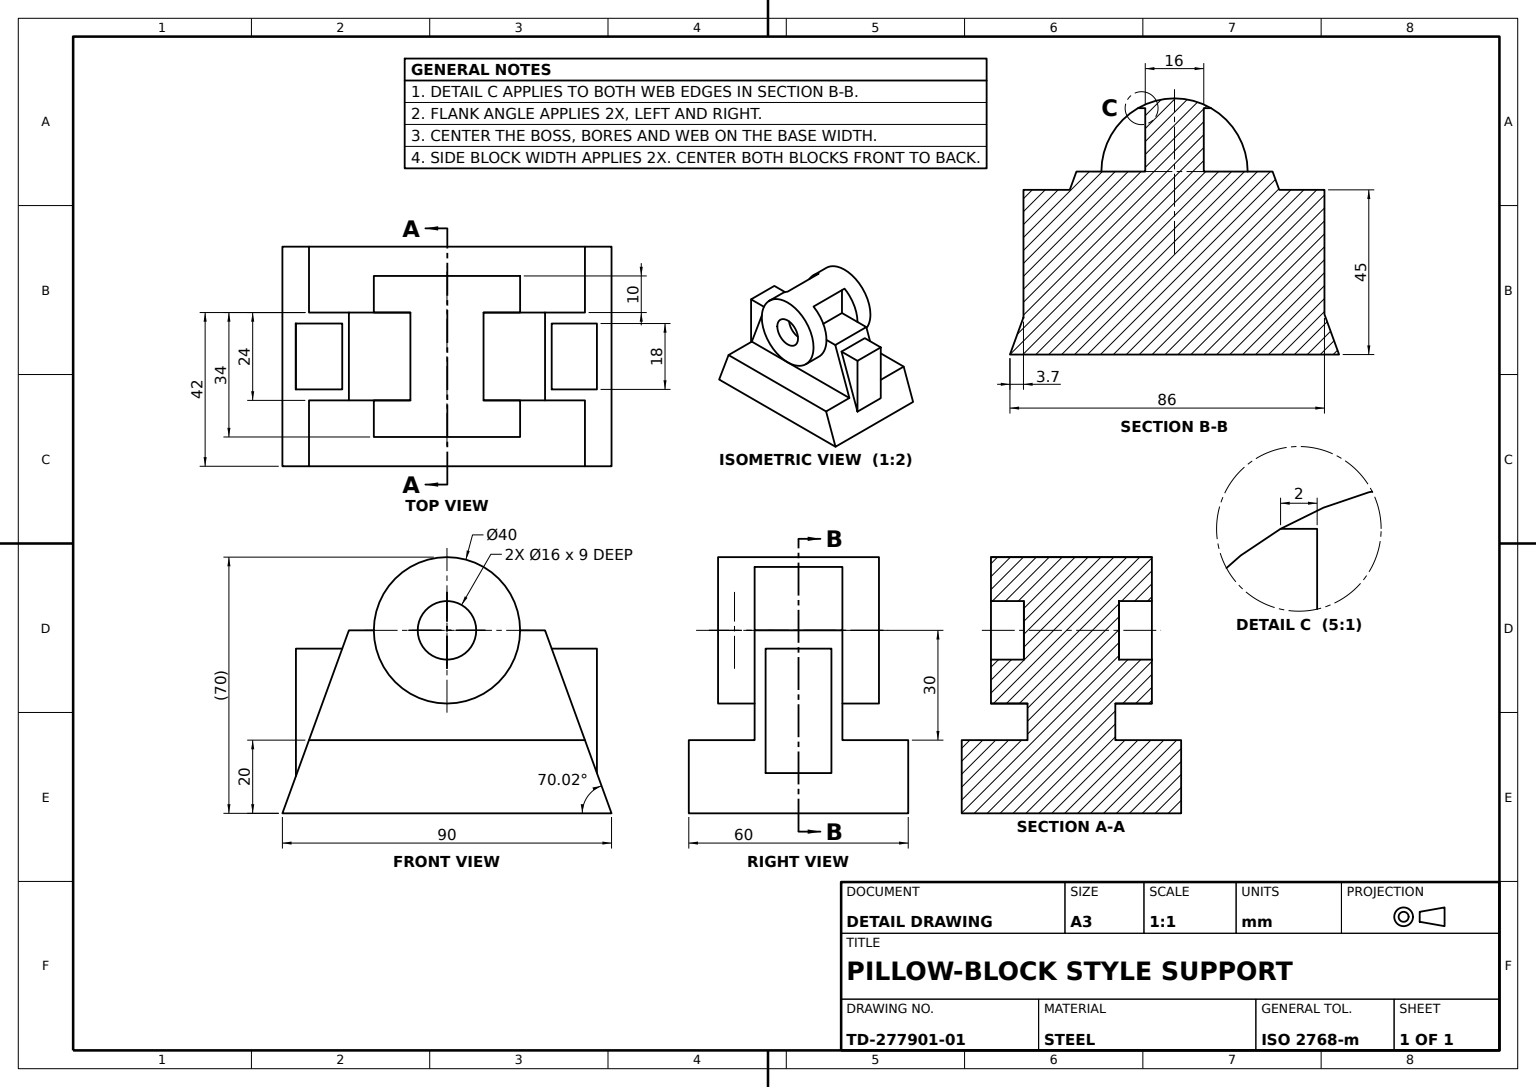
SolidWorks part; units mm, degrees
material "Plain Carbon Steel"
ref_plane "Front Plane" through (0, 0, 0) normal (0, 0, 1) x (1, 0, 0)
ref_plane "Top Plane" through (0, 0, 0) normal (0, 1, 0) x (1, 0, 0)
ref_plane "Right Plane" through (0, 0, 0) normal (1, 0, 0) x (0, 0, -1)
sketch "Base Trapezoid Sketch" plane through (0, 0, 0) normal (0, 0, 1) x (1, 0, 0)
  line L0 (0, 0) -> (90, 0)
  line L1 (90, 0) -> (90, 20)
  line L2 (90, 20) -> (0, 20)
  line L3 (0, 20) -> (0, 0)
  dimension "D1" = 90
  dimension "D2" = 20
extrude "Trapezoid Base" add sketch "Base Trapezoid Sketch" along normal blind 60
sketch "Support Profile Sketch" plane through (0, 0, 60) normal (0, 0, 1) x (1, 0, 0)
  line L0 (45, 20) -> (7.2727, 20)
  line L1 (90, 20) -> (0, 20) construction
  line L2 (45, 55) -> (20, 55)
  line L3 (20, 55) -> (7.2727, 20)
  line L4 (45, 55) -> (70, 55)
  line L5 (70, 55) -> (82.7273, 20)
  line L6 (45, 20) -> (82.7273, 20)
  line L7 (0, 20) -> (0, 0) construction
  line L8 (0, 0) -> (90, 0) construction
  dimension "D1" = 7.2727
  dimension "D2" = 20
  dimension "D3" = 55
extrude "Cylinder Support" add sketch "Support Profile Sketch" against normal blind 42
sketch "Support Notch Sketch" plane through (0, 0, 60) normal (0, 0, 1) x (1, 0, 0)
  line L0 (7.2727, 20) -> (20, 55)
  line L1 (20, 55) -> (70, 55)
  line L2 (70, 55) -> (82.7273, 20)
  line L3 (82.7273, 20) -> (7.2727, 20)
extrude "Support Notch Cut" cut sketch "Support Notch Sketch" against normal blind 18
sketch "Support Relief Sketch" plane through (0, 0, 42) normal (0, 0, 1) x (1, 0, 0)
  line L2 (45, 50) -> (71.8182, 50)
  line L3 (82.7273, 20) -> (70, 55) construction
  line L5 (45, 50) -> (18.1818, 50)
  line L6 (20, 55) -> (7.2727, 20) construction
  line L7 (18.1818, 50) -> (20, 55)
  line L8 (20, 55) -> (70, 55)
  line L9 (70, 55) -> (20, 55) construction
  line L10 (70, 55) -> (71.8182, 50)
  dimension "D1" = 10.9091
extrude "Support Relief Cut" cut sketch "Support Relief Sketch" against normal blind 24
sketch "Through Profile Sketch" plane through (0, 0, 60) normal (0, 0, 1) x (1, 0, 0)
  line L0 (0, 20) -> (7.2727, 20)
  line L1 (0, 20) -> (0, 0) construction
  line L2 (7.2727, 20) -> (0, 0)
  line L3 (90, 20) -> (82.7273, 20)
  line L4 (82.7273, 20) -> (90, 0)
  line L5 (90, 0) -> (90, 20)
  line M1 (90, 20) -> (0, 20)
  line M2 (0, 20) -> (0, 0)
  line M4 (90, 0) -> (90, 20)
extrude "Through Profile Cut" cut sketch "Through Profile Sketch" against normal blind 60 contours L2 M1 M2 | L4 M1 M4
sketch "Cylinder Sketch Ø40" plane through (0, 0, 42) normal (0, 0, 1) x (1, 0, 0)
  line L0 (18.1818, 50) -> (71.8182, 50) construction
  circle A0 centre (45, 50) radius 20
  dimension "D1" = 40
  dimension "D2" = 40
extrude "Cylinder Ø40" add sketch "Cylinder Sketch Ø40" against normal blind 34
sketch "Cylinder Extension Sketch" plane through (0, 0, 42) normal (0, 0, 1) x (1, 0, 0)
  circle A0 centre (45, 50) radius 20
  dimension "D1" = 40
  dimension "D2" = 40
extrude "Cylinder Extension Ø40" add sketch "Cylinder Extension Sketch" along normal blind 10
sketch "Front Bore Sketch Ø16" plane through (0, 0, 52) normal (0, 0, 1) x (1, 0, 0)
  circle A0 centre (45, 50) radius 8
  dimension "D1" = 16
  dimension "D2" = 16
extrude "Front Bore Ø16" cut sketch "Front Bore Sketch Ø16" against normal blind 10
sketch "Rear Bore Sketch" plane through (0, 0, 8) normal (0, 0, -1) x (-1, 0, 0)
  circle A0 centre (-45, 50) radius 8
  dimension "D1" = 16
extrude "Rear Bore" cut sketch "Rear Bore Sketch" against normal blind 10
ref_plane "Side Block Plane" through (0, 0, 0) normal (1, 0, 0) x (0, 0, -1)
sketch "Side Block Sketch" plane through (0, 0, 0) normal (1, 0, 0) x (0, 0, -1)
  line L2 (-30, 45) -> (-39, 45)
  line L3 (-39, 45) -> (-39, 10)
  line L4 (-39, 10) -> (-21, 10)
  line L5 (-21, 10) -> (-21, 45)
  line L6 (-21, 45) -> (-30, 45)
  dimension "D1" = 18
  dimension "D2" = 35
  dimension "D3" = 30
  dimension "D4" = 10
extrude "Side Blocks" add sketch "Side Block Sketch" along normal blind 86
sketch "Block Trim Sketch" plane through (0, 0, 0) normal (-1, 0, 0) x (0, 0, 1)
  line L0 (21, 45) -> (39, 45)
  line L1 (39, 45) -> (39, 10)
  line L2 (39, 10) -> (21, 10)
  line L3 (21, 10) -> (21, 45)
extrude "Block Trim Cut" cut sketch "Block Trim Sketch" against normal blind 3.7
ref_plane "Plane2" through (0, 50, 0) normal (0, 1, 0) x (1, 0, 0)
ref_plane "4" through (0, 70, 0) normal (0, 1, 0) x (1, 0, 0)
ref_plane "Plane4" through (0, 65, 0) normal (0, 1, 0) x (1, 0, 0)
ref_plane "Plane5" through (0, 50, 0) normal (0, 1, 0) x (1, 0, 0)
ref_plane "Slot A Plane" through (65, 0, 0) normal (1, 0, 0) x (0, 0, -1)
sketch "Slot A Sketch" plane through (65, 0, 0) normal (1, 0, 0) x (0, 0, -1)
  line L2 (-8, 70) -> (-52, 70) construction
  line L3 (-42, 70) -> (-18, 70)
  line L4 (-18, 70) -> (-18, 50)
  line L5 (-18, 50) -> (-42, 50)
  line L6 (-42, 70) -> (-42, 50)
extrude "Slot A Cut" cut sketch "Slot A Sketch" against normal blind 10
ref_plane "Slot B Plane" through (25, 0, 0) normal (1, 0, 0) x (0, 0, -1)
sketch "Slot B Sketch" plane through (25, 0, 0) normal (1, 0, 0) x (0, 0, -1)
  line L0 (-18, 50) -> (-18, 70)
  line L1 (-8, 70) -> (-52, 70) construction
  line L2 (-18, 70) -> (-42, 70)
  line L3 (-42, 70) -> (-42, 50)
  line L4 (-42, 50) -> (-18, 50)
extrude "Slot B Cut" cut sketch "Slot B Sketch" along normal blind 10
sketch "Front Bore Fill Sketch" plane through (0, 0, 42) normal (0, 0, 1) x (1, 0, 0)
  circle A0 centre (45, 50) radius 8
  dimension "D1" = 16
extrude "Front Bore Fill" add sketch "Front Bore Fill Sketch" along normal blind 10
sketch "Rear Bore Fill Sketch" plane through (0, 0, 18) normal (0, 0, -1) x (-1, 0, 0)
  circle A1 centre (-45, 50) radius 8
  dimension "D1" = 16
extrude "Rear Bore Fill" add sketch "Rear Bore Fill Sketch" along normal blind 10
sketch "Slot B Floor Sketch" plane through (35, 0, 0) normal (-1, 0, 0) x (0, 0, 1)
  line L0 (18, 67.3205) -> (42, 67.3205)
  line L1 (42, 67.3205) -> (42, 50)
  line L2 (42, 50) -> (18, 50)
  line L3 (18, 50) -> (18, 67.3205)
extrude "Slot B Floor Cut" cut sketch "Slot B Floor Sketch" against normal blind 2
sketch "Slot A Floor Sketch" plane through (55, 0, 0) normal (1, 0, 0) x (0, 0, -1)
  line L0 (-42, 67.3205) -> (-18, 67.3205)
  line L1 (-18, 67.3205) -> (-18, 50)
  line L2 (-18, 50) -> (-42, 50)
  line L3 (-42, 50) -> (-42, 67.3205)
extrude "Slot A Floor Cut" cut sketch "Slot A Floor Sketch" against normal blind 2
sketch "Front Bore Recut Sketch" plane through (0, 0, 52) normal (0, 0, 1) x (1, 0, 0)
  circle A0 centre (45, 50) radius 8
  dimension "D1" = 16
extrude "Front Bore Recut" cut sketch "Front Bore Recut Sketch" against normal blind 9
sketch "Rear Bore Recut Sketch" plane through (0, 0, 8) normal (0, 0, -1) x (-1, 0, 0)
  circle A0 centre (-45, 50) radius 8
  dimension "D1" = 16
extrude "Rear Bore Recut" cut sketch "Rear Bore Recut Sketch" against normal blind 9
